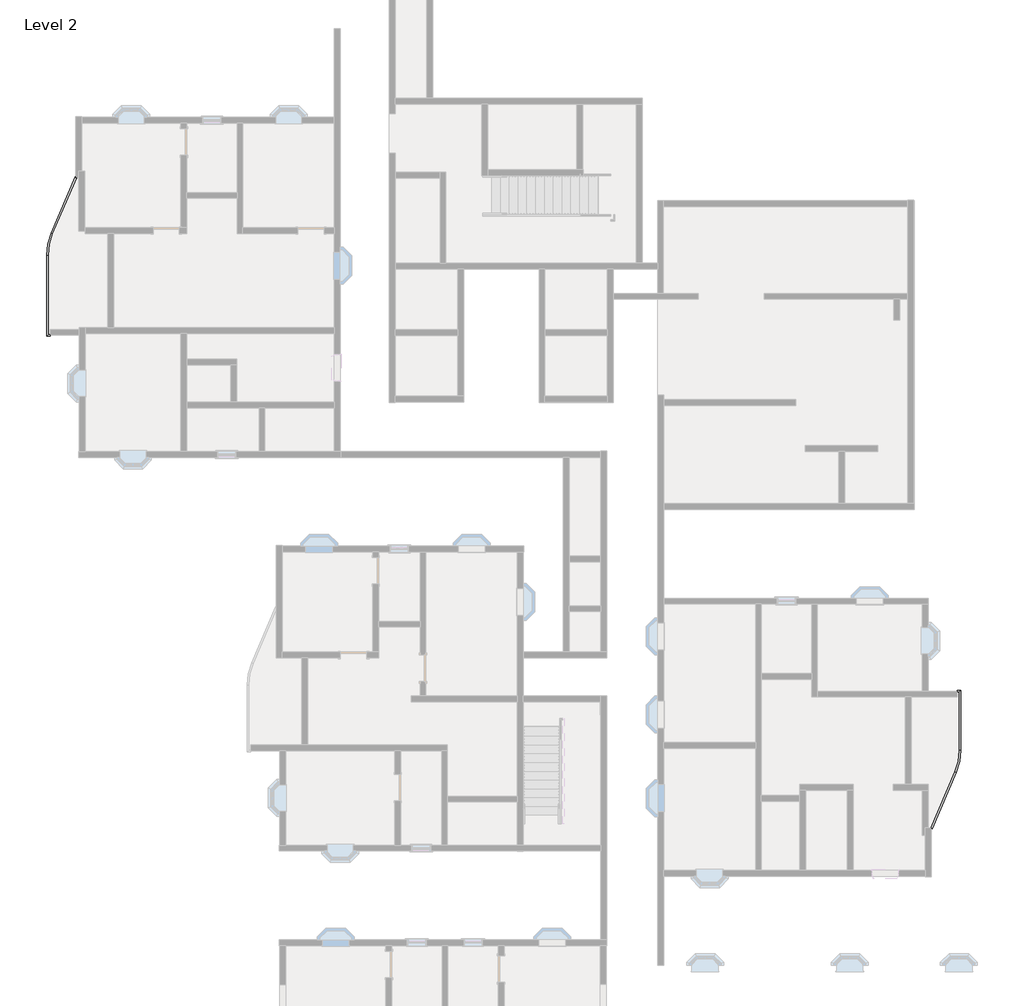
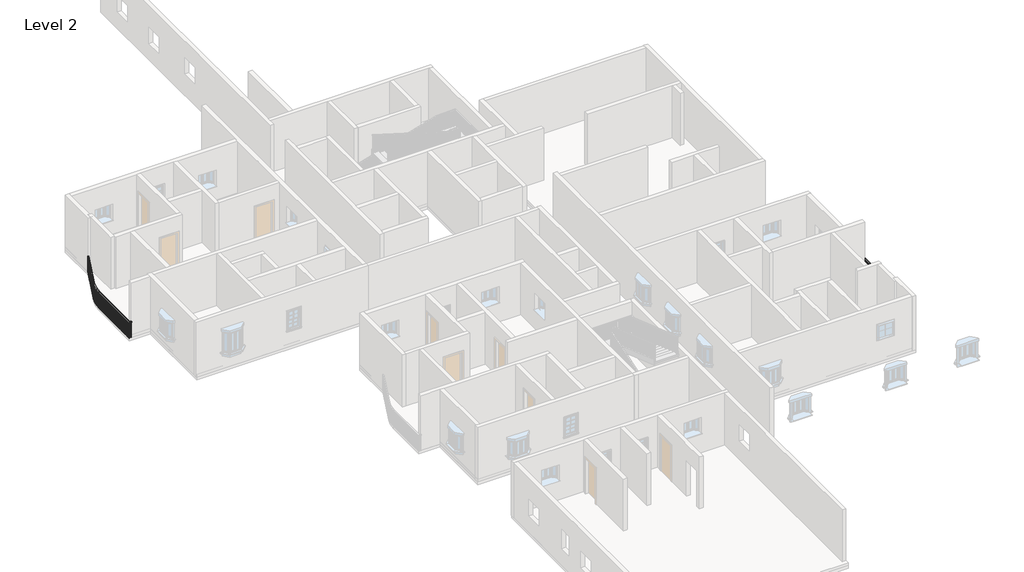
# One storey, part 9 of 14: 2 railings.
"""IFC4 building model written with IfcOpenShell, lengths in millimetres."""

from ifc_helpers import new_model, si_unit, frame, origin, place, context, project, spatial, polyline, circle_curve, outline, extrude, element, save
from ifc_brep_helpers import plane_surface, cylinder_surface, revolved_surface, advanced_brep

model = new_model("IFC4")

# Units and contexts
model_context = context("Model", 3, world=origin())
ifc_project = project(units=[si_unit("LENGTHUNIT", "METRE", prefix="MILLI")], contexts=[model_context])

# Site, building, storey
site = spatial("IfcSite", under=ifc_project)
building = spatial("IfcBuilding", under=site)
storey = spatial("IfcBuildingStorey", under=building, Name="Level 2", Elevation=3048.0)

# Railings
placement = place(None, origin())
element("IfcRailing", 1, ObjectType="Handrail - Rectangular", at=placement, inside=storey, context=model_context, shape_type="SolidModel", body=[
    advanced_brep(
    [(-19327.739878, 12446.0257339, 3962.4), (-19327.739878, 12446.0257339, 3911.6), (-19374.4383922, 12466.022953, 3911.6), (-19374.4383922, 12466.022953, 3962.4), (-20162.483418, 10496.6905323, 3962.4), (-20162.483418, 10496.6905323, 3911.6), (-20209.1819322, 10516.6877514, 3911.6), (-20209.1819322, 10516.6877514, 3962.4), (-20316.2891351, 9746.7948172, 3911.6), (-20316.2891351, 9746.7948172, 3962.4), (-20367.0891351, 9746.7948172, 3911.6), (-20367.0891351, 9746.7948172, 3962.4), (-20316.2891351, 7005.2583494, 3962.4), (-20316.2891351, 7005.2583494, 3911.6), (-20367.0891351, 6954.4583494, 3911.6), (-20367.0891351, 6954.4583494, 3962.4), (-20240.0891351, 7005.2583494, 3962.4), (-20240.0891351, 6954.4583494, 3962.4), (-20240.0891351, 6954.4583494, 3911.6), (-20240.0891351, 7005.2583494, 3911.6)],
    [
        (0, 1),
        (1, 2),
        (2, 3),
        (3, 0),
        (0, 4),
        (4, 5),
        (5, 1),
        (5, 6),
        (6, 2),
        (6, 7),
        (7, 3),
        (7, 4),
        (8, 5, circle_curve(frame((-18411.2891351, 9746.7948172, 3911.6), z_axis=(0.0, 0.0, -1.0), x_axis=(-0.9192620907623915, 0.3936460446735831, 0.0)), 1905.0)),
        (4, 9, circle_curve(frame((-18411.2891351, 9746.7948172, 3962.4), z_axis=(0.0, 0.0, 1.0), x_axis=(-0.9192620907623915, 0.3936460446735831, 0.0)), 1905.0)),
        (9, 8),
        (10, 6, circle_curve(frame((-18411.2891351, 9746.7948172, 3911.6), z_axis=(0.0, 0.0, -1.0), x_axis=(-0.9192620907623915, 0.3936460446735831, 0.0)), 1955.8)),
        (8, 10),
        (11, 7, circle_curve(frame((-18411.2891351, 9746.7948172, 3962.4), z_axis=(0.0, 0.0, -1.0), x_axis=(-0.9192620907623915, 0.3936460446735831, 0.0)), 1955.8)),
        (10, 11),
        (11, 9),
        (9, 12),
        (12, 13),
        (13, 8),
        (13, 14),
        (14, 10),
        (14, 15),
        (15, 11),
        (15, 12),
        (16, 17),
        (17, 18),
        (18, 19),
        (19, 16),
        (12, 16),
        (19, 13),
        (18, 14),
        (17, 15),
    ],
    [
        plane_surface(frame((-19351.0891351, 12456.0243434, 3962.4), z_axis=(0.3936460446735829, 0.9192620907623917, 0.0), x_axis=(0.9192620907623917, -0.3936460446735829, 0.0))),
        plane_surface(frame((-19327.739878, 12446.0257339, 3962.4), z_axis=(0.9192620907623913, -0.3936460446735837, 0.0), x_axis=(-0.3936460446735837, -0.9192620907623913, 0.0))),
        plane_surface(frame((-19327.739878, 12446.0257339, 3911.6), z_axis=(0.0, 0.0, -1.0), x_axis=(-0.3936460446735837, -0.9192620907623913, 0.0))),
        plane_surface(frame((-19374.4383922, 12466.022953, 3911.6), z_axis=(-0.9192620907623915, 0.3936460446735834, 0.0), x_axis=(-0.3936460446735834, -0.9192620907623915, 0.0))),
        plane_surface(frame((-19374.4383922, 12466.022953, 3962.4), z_axis=(0.0, 0.0, 1.0000000000000002), x_axis=(-0.3936460446735834, -0.9192620907623915, 0.0))),
        revolved_surface(polyline([(-20162.483418002357, 10496.690532303175, 3962.4), (-20162.483418002357, 10496.690532303175, 3911.6)]), (-18411.2891351, 9746.7948172, 3962.4), (0.0, 0.0, 1.0)),
        plane_surface(frame((-18411.2891351, 9746.7948172, 3911.6), z_axis=(0.0, 0.0, -1.0000000000000002), x_axis=(-0.9192620907623916, 0.39364604467358316, 0.0))),
        cylinder_surface(frame((-18411.2891351, 9746.7948172, 3962.4), z_axis=(0.0, 0.0, 1.0), x_axis=(-0.9192620907623915, 0.3936460446735831, 0.0)), 1955.8),
        plane_surface(frame((-18411.2891351, 9746.7948172, 3962.4), z_axis=(0.0, 0.0, 1.0000000000000002), x_axis=(-0.9192620907623916, 0.39364604467358316, 0.0))),
        plane_surface(frame((-20316.2891351, 9746.7948172, 3962.4), z_axis=(1.0, 0.0, 0.0), x_axis=(0.0, -1.0, 0.0))),
        plane_surface(frame((-20316.2891351, 9746.7948172, 3911.6), z_axis=(0.0, 0.0, -1.0), x_axis=(0.0, -1.0, 0.0))),
        plane_surface(frame((-20367.0891351, 9746.7948172, 3911.6), z_axis=(-1.0, 0.0, 0.0), x_axis=(0.0, -1.0, 0.0))),
        plane_surface(frame((-20367.0891351, 9746.7948172, 3962.4), z_axis=(0.0, 0.0, 1.0), x_axis=(0.0, -1.0, 0.0))),
        plane_surface(frame((-20240.0891351, 6979.8583494, 3962.4), z_axis=(1.0, 0.0, 0.0), x_axis=(0.0, 1.0, 0.0))),
        plane_surface(frame((-20316.2891351, 7005.2583494, 3962.4), z_axis=(0.0, 1.0, 0.0), x_axis=(1.0, 0.0, 0.0))),
        plane_surface(frame((-20316.2891351, 7005.2583494, 3911.6), z_axis=(0.0, 0.0, -1.0), x_axis=(1.0, 0.0, 0.0))),
        plane_surface(frame((-20367.0891351, 6954.4583494, 3911.6), z_axis=(0.0, -1.0, 0.0), x_axis=(1.0, 0.0, 0.0))),
        plane_surface(frame((-20367.0891351, 6954.4583494, 3962.4), z_axis=(0.0, 0.0, 1.0), x_axis=(1.0, 0.0, 0.0))),
    ],
    [
        (0, [[1, 2, 3, 4]]),
        (1, [[-1, 5, 6, 7]]),
        (2, [[-2, -7, 8, 9]]),
        (3, [[-3, -9, 10, 11]]),
        (4, [[-4, -11, 12, -5]]),
        (5, [[13, -6, 14, 15]]),
        (6, [[16, -8, -13, 17]]),
        (7, [[18, -10, -16, 19]]),
        (8, [[-14, -12, -18, 20]]),
        (9, [[-15, 21, 22, 23]]),
        (10, [[-17, -23, 24, 25]]),
        (11, [[-19, -25, 26, 27]]),
        (12, [[-20, -27, 28, -21]]),
        (13, [[29, 30, 31, 32]]),
        (14, [[-22, 33, -32, 34]]),
        (15, [[-24, -34, -31, 35]]),
        (16, [[-26, -35, -30, 36]]),
        (17, [[-28, -36, -29, -33]]),
    ],
),
    extrude(outline(polyline([(-20351.2141351, 7013.1198172), (-20332.1641351, 7013.1198172), (-20332.1641351, 6994.0698172), (-20351.2141351, 6994.0698172), (-20351.2141351, 7013.1198172)])), frame((0.0, 0.0, 3048.0), z_axis=(0.0, 0.0, 1.0), x_axis=(1.0, 0.0, 0.0)), (0.0, 0.0, 1.0), 863.6),
    extrude(outline(polyline([(-20351.2141351, 7114.7198172), (-20332.1641351, 7114.7198172), (-20332.1641351, 7095.6698172), (-20351.2141351, 7095.6698172), (-20351.2141351, 7114.7198172)])), frame((0.0, 0.0, 3048.0), z_axis=(0.0, 0.0, 1.0), x_axis=(1.0, 0.0, 0.0)), (0.0, 0.0, 1.0), 863.6),
    extrude(outline(polyline([(-20351.2141351, 7216.3198172), (-20332.1641351, 7216.3198172), (-20332.1641351, 7197.2698172), (-20351.2141351, 7197.2698172), (-20351.2141351, 7216.3198172)])), frame((0.0, 0.0, 3048.0), z_axis=(0.0, 0.0, 1.0), x_axis=(1.0, 0.0, 0.0)), (0.0, 0.0, 1.0), 863.6),
    extrude(outline(polyline([(-20351.2141351, 7317.9198172), (-20332.1641351, 7317.9198172), (-20332.1641351, 7298.8698172), (-20351.2141351, 7298.8698172), (-20351.2141351, 7317.9198172)])), frame((0.0, 0.0, 3048.0), z_axis=(0.0, 0.0, 1.0), x_axis=(1.0, 0.0, 0.0)), (0.0, 0.0, 1.0), 863.6),
    extrude(outline(polyline([(-20351.2141351, 7419.5198172), (-20332.1641351, 7419.5198172), (-20332.1641351, 7400.4698172), (-20351.2141351, 7400.4698172), (-20351.2141351, 7419.5198172)])), frame((0.0, 0.0, 3048.0), z_axis=(0.0, 0.0, 1.0), x_axis=(1.0, 0.0, 0.0)), (0.0, 0.0, 1.0), 863.6),
    extrude(outline(polyline([(-20351.2141351, 7521.1198172), (-20332.1641351, 7521.1198172), (-20332.1641351, 7502.0698172), (-20351.2141351, 7502.0698172), (-20351.2141351, 7521.1198172)])), frame((0.0, 0.0, 3048.0), z_axis=(0.0, 0.0, 1.0), x_axis=(1.0, 0.0, 0.0)), (0.0, 0.0, 1.0), 863.6),
    extrude(outline(polyline([(-20351.2141351, 7622.7198172), (-20332.1641351, 7622.7198172), (-20332.1641351, 7603.6698172), (-20351.2141351, 7603.6698172), (-20351.2141351, 7622.7198172)])), frame((0.0, 0.0, 3048.0), z_axis=(0.0, 0.0, 1.0), x_axis=(1.0, 0.0, 0.0)), (0.0, 0.0, 1.0), 863.6),
    extrude(outline(polyline([(-20351.2141351, 7724.3198172), (-20332.1641351, 7724.3198172), (-20332.1641351, 7705.2698172), (-20351.2141351, 7705.2698172), (-20351.2141351, 7724.3198172)])), frame((0.0, 0.0, 3048.0), z_axis=(0.0, 0.0, 1.0), x_axis=(1.0, 0.0, 0.0)), (0.0, 0.0, 1.0), 863.6),
    extrude(outline(polyline([(-20351.2141351, 7825.9198172), (-20332.1641351, 7825.9198172), (-20332.1641351, 7806.8698172), (-20351.2141351, 7806.8698172), (-20351.2141351, 7825.9198172)])), frame((0.0, 0.0, 3048.0), z_axis=(0.0, 0.0, 1.0), x_axis=(1.0, 0.0, 0.0)), (0.0, 0.0, 1.0), 863.6),
    extrude(outline(polyline([(-20351.2141351, 7927.5198172), (-20332.1641351, 7927.5198172), (-20332.1641351, 7908.4698172), (-20351.2141351, 7908.4698172), (-20351.2141351, 7927.5198172)])), frame((0.0, 0.0, 3048.0), z_axis=(0.0, 0.0, 1.0), x_axis=(1.0, 0.0, 0.0)), (0.0, 0.0, 1.0), 863.6),
    extrude(outline(polyline([(-20351.2141351, 8029.1198172), (-20332.1641351, 8029.1198172), (-20332.1641351, 8010.0698172), (-20351.2141351, 8010.0698172), (-20351.2141351, 8029.1198172)])), frame((0.0, 0.0, 3048.0), z_axis=(0.0, 0.0, 1.0), x_axis=(1.0, 0.0, 0.0)), (0.0, 0.0, 1.0), 863.6),
    extrude(outline(polyline([(-20351.2141351, 8130.7198172), (-20332.1641351, 8130.7198172), (-20332.1641351, 8111.6698172), (-20351.2141351, 8111.6698172), (-20351.2141351, 8130.7198172)])), frame((0.0, 0.0, 3048.0), z_axis=(0.0, 0.0, 1.0), x_axis=(1.0, 0.0, 0.0)), (0.0, 0.0, 1.0), 863.6),
    extrude(outline(polyline([(-20351.2141351, 8232.3198172), (-20332.1641351, 8232.3198172), (-20332.1641351, 8213.2698172), (-20351.2141351, 8213.2698172), (-20351.2141351, 8232.3198172)])), frame((0.0, 0.0, 3048.0), z_axis=(0.0, 0.0, 1.0), x_axis=(1.0, 0.0, 0.0)), (0.0, 0.0, 1.0), 863.6),
    extrude(outline(polyline([(-20351.2141351, 8333.9198172), (-20332.1641351, 8333.9198172), (-20332.1641351, 8314.8698172), (-20351.2141351, 8314.8698172), (-20351.2141351, 8333.9198172)])), frame((0.0, 0.0, 3048.0), z_axis=(0.0, 0.0, 1.0), x_axis=(1.0, 0.0, 0.0)), (0.0, 0.0, 1.0), 863.6),
    extrude(outline(polyline([(-20351.2141351, 8435.5198172), (-20332.1641351, 8435.5198172), (-20332.1641351, 8416.4698172), (-20351.2141351, 8416.4698172), (-20351.2141351, 8435.5198172)])), frame((0.0, 0.0, 3048.0), z_axis=(0.0, 0.0, 1.0), x_axis=(1.0, 0.0, 0.0)), (0.0, 0.0, 1.0), 863.6),
    extrude(outline(polyline([(-20351.2141351, 8537.1198172), (-20332.1641351, 8537.1198172), (-20332.1641351, 8518.0698172), (-20351.2141351, 8518.0698172), (-20351.2141351, 8537.1198172)])), frame((0.0, 0.0, 3048.0), z_axis=(0.0, 0.0, 1.0), x_axis=(1.0, 0.0, 0.0)), (0.0, 0.0, 1.0), 863.6),
    extrude(outline(polyline([(-20351.2141351, 8638.7198172), (-20332.1641351, 8638.7198172), (-20332.1641351, 8619.6698172), (-20351.2141351, 8619.6698172), (-20351.2141351, 8638.7198172)])), frame((0.0, 0.0, 3048.0), z_axis=(0.0, 0.0, 1.0), x_axis=(1.0, 0.0, 0.0)), (0.0, 0.0, 1.0), 863.6),
    extrude(outline(polyline([(-20351.2141351, 8740.3198172), (-20332.1641351, 8740.3198172), (-20332.1641351, 8721.2698172), (-20351.2141351, 8721.2698172), (-20351.2141351, 8740.3198172)])), frame((0.0, 0.0, 3048.0), z_axis=(0.0, 0.0, 1.0), x_axis=(1.0, 0.0, 0.0)), (0.0, 0.0, 1.0), 863.6),
    extrude(outline(polyline([(-20351.2141351, 8841.9198172), (-20332.1641351, 8841.9198172), (-20332.1641351, 8822.8698172), (-20351.2141351, 8822.8698172), (-20351.2141351, 8841.9198172)])), frame((0.0, 0.0, 3048.0), z_axis=(0.0, 0.0, 1.0), x_axis=(1.0, 0.0, 0.0)), (0.0, 0.0, 1.0), 863.6),
    extrude(outline(polyline([(-20351.2141351, 8943.5198172), (-20332.1641351, 8943.5198172), (-20332.1641351, 8924.4698172), (-20351.2141351, 8924.4698172), (-20351.2141351, 8943.5198172)])), frame((0.0, 0.0, 3048.0), z_axis=(0.0, 0.0, 1.0), x_axis=(1.0, 0.0, 0.0)), (0.0, 0.0, 1.0), 863.6),
    extrude(outline(polyline([(-20351.2141351, 9045.1198172), (-20332.1641351, 9045.1198172), (-20332.1641351, 9026.0698172), (-20351.2141351, 9026.0698172), (-20351.2141351, 9045.1198172)])), frame((0.0, 0.0, 3048.0), z_axis=(0.0, 0.0, 1.0), x_axis=(1.0, 0.0, 0.0)), (0.0, 0.0, 1.0), 863.6),
    extrude(outline(polyline([(-20351.2141351, 9146.7198172), (-20332.1641351, 9146.7198172), (-20332.1641351, 9127.6698172), (-20351.2141351, 9127.6698172), (-20351.2141351, 9146.7198172)])), frame((0.0, 0.0, 3048.0), z_axis=(0.0, 0.0, 1.0), x_axis=(1.0, 0.0, 0.0)), (0.0, 0.0, 1.0), 863.6),
    extrude(outline(polyline([(-20351.2141351, 9248.3198172), (-20332.1641351, 9248.3198172), (-20332.1641351, 9229.2698172), (-20351.2141351, 9229.2698172), (-20351.2141351, 9248.3198172)])), frame((0.0, 0.0, 3048.0), z_axis=(0.0, 0.0, 1.0), x_axis=(1.0, 0.0, 0.0)), (0.0, 0.0, 1.0), 863.6),
    extrude(outline(polyline([(-20351.2141351, 9349.9198172), (-20332.1641351, 9349.9198172), (-20332.1641351, 9330.8698172), (-20351.2141351, 9330.8698172), (-20351.2141351, 9349.9198172)])), frame((0.0, 0.0, 3048.0), z_axis=(0.0, 0.0, 1.0), x_axis=(1.0, 0.0, 0.0)), (0.0, 0.0, 1.0), 863.6),
    extrude(outline(polyline([(-20351.2141351, 9451.5198172), (-20332.1641351, 9451.5198172), (-20332.1641351, 9432.4698172), (-20351.2141351, 9432.4698172), (-20351.2141351, 9451.5198172)])), frame((0.0, 0.0, 3048.0), z_axis=(0.0, 0.0, 1.0), x_axis=(1.0, 0.0, 0.0)), (0.0, 0.0, 1.0), 863.6),
    extrude(outline(polyline([(-20351.2141351, 9553.1198172), (-20332.1641351, 9553.1198172), (-20332.1641351, 9534.0698172), (-20351.2141351, 9534.0698172), (-20351.2141351, 9553.1198172)])), frame((0.0, 0.0, 3048.0), z_axis=(0.0, 0.0, 1.0), x_axis=(1.0, 0.0, 0.0)), (0.0, 0.0, 1.0), 863.6),
    extrude(outline(polyline([(-20351.2141351, 9654.7198172), (-20332.1641351, 9654.7198172), (-20332.1641351, 9635.6698172), (-20351.2141351, 9635.6698172), (-20351.2141351, 9654.7198172)])), frame((0.0, 0.0, 3048.0), z_axis=(0.0, 0.0, 1.0), x_axis=(1.0, 0.0, 0.0)), (0.0, 0.0, 1.0), 863.6),
    extrude(outline(polyline([(-20349.6005818, 9826.4720848), (-20330.5630441, 9825.7831307), (-20331.2519982, 9806.745593), (-20350.289536, 9807.4345471), (-20349.6005818, 9826.4720848)])), frame((0.0, 0.0, 3048.0), z_axis=(0.0, 0.0, 1.0), x_axis=(1.0, 0.0, 0.0)), (0.0, 0.0, 1.0), 863.6),
    extrude(outline(polyline([(-20342.724955, 9928.3310534), (-20323.750023, 9926.6415402), (-20325.4395363, 9907.6666081), (-20344.4144683, 9909.3561214), (-20342.724955, 9928.3310534)])), frame((0.0, 0.0, 3048.0), z_axis=(0.0, 0.0, 1.0), x_axis=(1.0, 0.0, 0.0)), (0.0, 0.0, 1.0), 863.6),
    extrude(outline(polyline([(-20330.5003254, 10029.6872677), (-20311.6405491, 10027.0018743), (-20314.3259425, 10008.142098), (-20333.1857188, 10010.8274914), (-20330.5003254, 10029.6872677)])), frame((0.0, 0.0, 3048.0), z_axis=(0.0, 0.0, 1.0), x_axis=(1.0, 0.0, 0.0)), (0.0, 0.0, 1.0), 863.6),
    extrude(outline(polyline([(-20312.9605484, 10130.2600272), (-20294.2681589, 10126.5861907), (-20297.9419954, 10107.8938012), (-20316.6343849, 10111.5676377), (-20312.9605484, 10130.2600272)])), frame((0.0, 0.0, 3048.0), z_axis=(0.0, 0.0, 1.0), x_axis=(1.0, 0.0, 0.0)), (0.0, 0.0, 1.0), 863.6),
    extrude(outline(polyline([(-20290.1541995, 10229.7708014), (-20271.6809643, 10225.1186963), (-20276.3330693, 10206.6454611), (-20294.8063045, 10211.2975662), (-20290.1541995, 10229.7708014)])), frame((0.0, 0.0, 3048.0), z_axis=(0.0, 0.0, 1.0), x_axis=(1.0, 0.0, 0.0)), (0.0, 0.0, 1.0), 863.6),
    extrude(outline(polyline([(-20262.1444395, 10327.9440008), (-20243.9415192, 10322.3265109), (-20249.5590091, 10304.1235906), (-20267.7619294, 10309.7410805), (-20262.1444395, 10327.9440008)])), frame((0.0, 0.0, 3048.0), z_axis=(0.0, 0.0, 1.0), x_axis=(1.0, 0.0, 0.0)), (0.0, 0.0, 1.0), 863.6),
    extrude(outline(polyline([(-20229.0088399, 10424.5077402), (-20211.1266465, 10417.9404228), (-20217.693964, 10400.0582293), (-20235.5761574, 10406.6255468), (-20229.0088399, 10424.5077402)])), frame((0.0, 0.0, 3048.0), z_axis=(0.0, 0.0, 1.0), x_axis=(1.0, 0.0, 0.0)), (0.0, 0.0, 1.0), 863.6),
    extrude(outline(polyline([(-20155.9843907, 10600.589225), (-20138.4724479, 10593.0902678), (-20145.9714051, 10575.578325), (-20163.4833479, 10583.0772822), (-20155.9843907, 10600.589225)])), frame((0.0, 0.0, 3048.0), z_axis=(0.0, 0.0, 1.0), x_axis=(1.0, 0.0, 0.0)), (0.0, 0.0, 1.0), 863.6),
    extrude(outline(polyline([(-20115.9899526, 10693.9862534), (-20098.4780098, 10686.4872963), (-20105.9769669, 10668.9753534), (-20123.4889098, 10676.4743106), (-20115.9899526, 10693.9862534)])), frame((0.0, 0.0, 3048.0), z_axis=(0.0, 0.0, 1.0), x_axis=(1.0, 0.0, 0.0)), (0.0, 0.0, 1.0), 863.6),
    extrude(outline(polyline([(-20075.9955145, 10787.3832818), (-20058.4835716, 10779.8843247), (-20065.9825288, 10762.3723818), (-20083.4944716, 10769.871339), (-20075.9955145, 10787.3832818)])), frame((0.0, 0.0, 3048.0), z_axis=(0.0, 0.0, 1.0), x_axis=(1.0, 0.0, 0.0)), (0.0, 0.0, 1.0), 863.6),
    extrude(outline(polyline([(-20036.0010763, 10880.7803103), (-20018.4891335, 10873.2813531), (-20025.9880906, 10855.7694103), (-20043.5000335, 10863.2683674), (-20036.0010763, 10880.7803103)])), frame((0.0, 0.0, 3048.0), z_axis=(0.0, 0.0, 1.0), x_axis=(1.0, 0.0, 0.0)), (0.0, 0.0, 1.0), 863.6),
    extrude(outline(polyline([(-19996.0066382, 10974.1773387), (-19978.4946954, 10966.6783815), (-19985.9936525, 10949.1664387), (-20003.5055953, 10956.6653958), (-19996.0066382, 10974.1773387)])), frame((0.0, 0.0, 3048.0), z_axis=(0.0, 0.0, 1.0), x_axis=(1.0, 0.0, 0.0)), (0.0, 0.0, 1.0), 863.6),
    extrude(outline(polyline([(-19956.0122, 11067.5743671), (-19938.5002572, 11060.0754099), (-19945.9992144, 11042.5634671), (-19963.5111572, 11050.0624243), (-19956.0122, 11067.5743671)])), frame((0.0, 0.0, 3048.0), z_axis=(0.0, 0.0, 1.0), x_axis=(1.0, 0.0, 0.0)), (0.0, 0.0, 1.0), 863.6),
    extrude(outline(polyline([(-19916.0177619, 11160.9713955), (-19898.5058191, 11153.4724384), (-19906.0047762, 11135.9604955), (-19923.5167191, 11143.4594527), (-19916.0177619, 11160.9713955)])), frame((0.0, 0.0, 3048.0), z_axis=(0.0, 0.0, 1.0), x_axis=(1.0, 0.0, 0.0)), (0.0, 0.0, 1.0), 863.6),
    extrude(outline(polyline([(-19876.0233238, 11254.3684239), (-19858.5113809, 11246.8694668), (-19866.0103381, 11229.357524), (-19883.5222809, 11236.8564811), (-19876.0233238, 11254.3684239)])), frame((0.0, 0.0, 3048.0), z_axis=(0.0, 0.0, 1.0), x_axis=(1.0, 0.0, 0.0)), (0.0, 0.0, 1.0), 863.6),
    extrude(outline(polyline([(-19836.0288856, 11347.7654524), (-19818.5169428, 11340.2664952), (-19826.0159, 11322.7545524), (-19843.5278428, 11330.2535095), (-19836.0288856, 11347.7654524)])), frame((0.0, 0.0, 3048.0), z_axis=(0.0, 0.0, 1.0), x_axis=(1.0, 0.0, 0.0)), (0.0, 0.0, 1.0), 863.6),
    extrude(outline(polyline([(-19796.0344475, 11441.1624808), (-19778.5225047, 11433.6635236), (-19786.0214618, 11416.1515808), (-19803.5334046, 11423.650538), (-19796.0344475, 11441.1624808)])), frame((0.0, 0.0, 3048.0), z_axis=(0.0, 0.0, 1.0), x_axis=(1.0, 0.0, 0.0)), (0.0, 0.0, 1.0), 863.6),
    extrude(outline(polyline([(-19756.0400094, 11534.5595092), (-19738.5280665, 11527.060552), (-19746.0270237, 11509.5486092), (-19763.5389665, 11517.0475664), (-19756.0400094, 11534.5595092)])), frame((0.0, 0.0, 3048.0), z_axis=(0.0, 0.0, 1.0), x_axis=(1.0, 0.0, 0.0)), (0.0, 0.0, 1.0), 863.6),
    extrude(outline(polyline([(-19716.0455712, 11627.9565376), (-19698.5336284, 11620.4575805), (-19706.0325855, 11602.9456376), (-19723.5445284, 11610.4445948), (-19716.0455712, 11627.9565376)])), frame((0.0, 0.0, 3048.0), z_axis=(0.0, 0.0, 1.0), x_axis=(1.0, 0.0, 0.0)), (0.0, 0.0, 1.0), 863.6),
    extrude(outline(polyline([(-19676.0511331, 11721.353566), (-19658.5391902, 11713.8546089), (-19666.0381474, 11696.3426661), (-19683.5500902, 11703.8416232), (-19676.0511331, 11721.353566)])), frame((0.0, 0.0, 3048.0), z_axis=(0.0, 0.0, 1.0), x_axis=(1.0, 0.0, 0.0)), (0.0, 0.0, 1.0), 863.6),
    extrude(outline(polyline([(-19636.0566949, 11814.7505945), (-19618.5447521, 11807.2516373), (-19626.0437093, 11789.7396945), (-19643.5556521, 11797.2386516), (-19636.0566949, 11814.7505945)])), frame((0.0, 0.0, 3048.0), z_axis=(0.0, 0.0, 1.0), x_axis=(1.0, 0.0, 0.0)), (0.0, 0.0, 1.0), 863.6),
    extrude(outline(polyline([(-19596.0622568, 11908.1476229), (-19578.550314, 11900.6486657), (-19586.0492711, 11883.1367229), (-19603.561214, 11890.6356801), (-19596.0622568, 11908.1476229)])), frame((0.0, 0.0, 3048.0), z_axis=(0.0, 0.0, 1.0), x_axis=(1.0, 0.0, 0.0)), (0.0, 0.0, 1.0), 863.6),
    extrude(outline(polyline([(-19556.0678187, 12001.5446513), (-19538.5558758, 11994.0456942), (-19546.054833, 11976.5337513), (-19563.5667758, 11984.0327085), (-19556.0678187, 12001.5446513)])), frame((0.0, 0.0, 3048.0), z_axis=(0.0, 0.0, 1.0), x_axis=(1.0, 0.0, 0.0)), (0.0, 0.0, 1.0), 863.6),
    extrude(outline(polyline([(-19516.0733805, 12094.9416797), (-19498.5614377, 12087.4427226), (-19506.0603948, 12069.9307797), (-19523.5723377, 12077.4297369), (-19516.0733805, 12094.9416797)])), frame((0.0, 0.0, 3048.0), z_axis=(0.0, 0.0, 1.0), x_axis=(1.0, 0.0, 0.0)), (0.0, 0.0, 1.0), 863.6),
    extrude(outline(polyline([(-19476.0789424, 12188.3387082), (-19458.5669996, 12180.839751), (-19466.0659567, 12163.3278082), (-19483.5778995, 12170.8267653), (-19476.0789424, 12188.3387082)])), frame((0.0, 0.0, 3048.0), z_axis=(0.0, 0.0, 1.0), x_axis=(1.0, 0.0, 0.0)), (0.0, 0.0, 1.0), 863.6),
    extrude(outline(polyline([(-19436.0845042, 12281.7357366), (-19418.5725614, 12274.2367794), (-19426.0715186, 12256.7248366), (-19443.5834614, 12264.2237937), (-19436.0845042, 12281.7357366)])), frame((0.0, 0.0, 3048.0), z_axis=(0.0, 0.0, 1.0), x_axis=(1.0, 0.0, 0.0)), (0.0, 0.0, 1.0), 863.6),
    extrude(outline(polyline([(-19396.0900661, 12375.132765), (-19378.5781233, 12367.6338078), (-19386.0770804, 12350.121865), (-19403.5890233, 12357.6208222), (-19396.0900661, 12375.132765)])), frame((0.0, 0.0, 3048.0), z_axis=(0.0, 0.0, 1.0), x_axis=(1.0, 0.0, 0.0)), (0.0, 0.0, 1.0), 863.6),
    extrude(outline(polyline([(-20351.2141351, 6989.3833494), (-20332.1641351, 6989.3833494), (-20332.1641351, 6970.3333494), (-20351.2141351, 6970.3333494), (-20351.2141351, 6989.3833494)])), frame((0.0, 0.0, 3048.0), z_axis=(0.0, 0.0, 1.0), x_axis=(1.0, 0.0, 0.0)), (0.0, 0.0, 1.0), 863.6),
    extrude(outline(polyline([(-20351.2141351, 9756.3198172), (-20332.1641351, 9756.3198172), (-20332.1641351, 9737.2698172), (-20351.2141351, 9737.2698172), (-20351.2141351, 9756.3198172)])), frame((0.0, 0.0, 3048.0), z_axis=(0.0, 0.0, 1.0), x_axis=(1.0, 0.0, 0.0)), (0.0, 0.0, 1.0), 863.6),
    extrude(outline(polyline([(-20190.839168, 10519.1945919), (-20173.3272251, 10511.6956347), (-20180.8261823, 10494.1836919), (-20198.3381251, 10501.682649), (-20190.839168, 10519.1945919)])), frame((0.0, 0.0, 3048.0), z_axis=(0.0, 0.0, 1.0), x_axis=(1.0, 0.0, 0.0)), (0.0, 0.0, 1.0), 863.6),
    extrude(outline(polyline([(-20259.1391351, 6970.3333494), (-20259.1391351, 6989.3833494), (-20240.0891351, 6989.3833494), (-20240.0891351, 6970.3333494), (-20259.1391351, 6970.3333494)])), frame((0.0, 0.0, 3048.0), z_axis=(0.0, 0.0, 1.0), x_axis=(1.0, 0.0, 0.0)), (0.0, 0.0, 1.0), 863.6),
    extrude(outline(polyline([(-19359.8451065, 12459.773822), (-19342.3331637, 12452.2748648), (-19349.8321209, 12434.762922), (-19367.3440637, 12442.2618792), (-19359.8451065, 12459.773822)])), frame((0.0, 0.0, 3048.0), z_axis=(0.0, 0.0, 1.0), x_axis=(1.0, 0.0, 0.0)), (0.0, 0.0, 1.0), 863.6),
])
element("IfcRailing", 2, ObjectType="Handrail - Rectangular", at=placement, inside=storey, context=model_context, shape_type="SolidModel", body=[
    advanced_brep(
    [(10250.7887952, -10096.81198, 3962.4), (10250.7887952, -10096.81198, 3911.6), (10297.4873094, -10116.8091991, 3911.6), (10297.4873094, -10116.8091991, 3962.4), (11085.5323352, -8147.4767784, 3962.4), (11085.5323352, -8147.4767784, 3911.6), (11132.2308494, -8167.4739975, 3911.6), (11132.2308494, -8167.4739975, 3962.4), (11239.3380523, -7397.5810633, 3911.6), (11239.3380523, -7397.5810633, 3962.4), (11290.1380523, -7397.5810633, 3911.6), (11290.1380523, -7397.5810633, 3962.4), (11239.3380523, -5378.0542694, 3962.4), (11239.3380523, -5378.0542694, 3911.6), (11290.1380523, -5327.2542694, 3911.6), (11290.1380523, -5327.2542694, 3962.4), (11163.1380523, -5378.0542694, 3962.4), (11163.1380523, -5327.2542694, 3962.4), (11163.1380523, -5327.2542694, 3911.6), (11163.1380523, -5378.0542694, 3911.6)],
    [
        (0, 1),
        (1, 2),
        (2, 3),
        (3, 0),
        (0, 4),
        (4, 5),
        (5, 1),
        (5, 6),
        (6, 2),
        (6, 7),
        (7, 3),
        (7, 4),
        (8, 5, circle_curve(frame((9334.3380523, -7397.5810633, 3911.6), z_axis=(0.0, 0.0, -1.0), x_axis=(0.9192620907624003, -0.3936460446735628, 0.0)), 1905.0)),
        (4, 9, circle_curve(frame((9334.3380523, -7397.5810633, 3962.4), z_axis=(0.0, 0.0, 1.0), x_axis=(0.9192620907624003, -0.3936460446735628, 0.0)), 1905.0)),
        (9, 8),
        (10, 6, circle_curve(frame((9334.3380523, -7397.5810633, 3911.6), z_axis=(0.0, 0.0, -1.0), x_axis=(0.9192620907624003, -0.3936460446735628, 0.0)), 1955.8)),
        (8, 10),
        (11, 7, circle_curve(frame((9334.3380523, -7397.5810633, 3962.4), z_axis=(0.0, 0.0, -1.0), x_axis=(0.9192620907624003, -0.3936460446735628, 0.0)), 1955.8)),
        (10, 11),
        (11, 9),
        (9, 12),
        (12, 13),
        (13, 8),
        (13, 14),
        (14, 10),
        (14, 15),
        (15, 11),
        (15, 12),
        (16, 17),
        (17, 18),
        (18, 19),
        (19, 16),
        (12, 16),
        (19, 13),
        (18, 14),
        (17, 15),
    ],
    [
        plane_surface(frame((10274.1380523, -10106.8105895, 3962.4), z_axis=(-0.3936460446735629, -0.9192620907624003, 0.0), x_axis=(0.9192620907624003, -0.3936460446735629, 0.0))),
        plane_surface(frame((10250.7887952, -10096.81198, 3962.4), z_axis=(-0.9192620907624004, 0.3936460446735625, 0.0), x_axis=(0.3936460446735625, 0.9192620907624004, 0.0))),
        plane_surface(frame((10250.7887952, -10096.81198, 3911.6), z_axis=(0.0, 0.0, -1.0), x_axis=(0.3936460446735625, 0.9192620907624004, 0.0))),
        plane_surface(frame((10297.4873094, -10116.8091991, 3911.6), z_axis=(0.9192620907624003, -0.3936460446735629, 0.0), x_axis=(0.3936460446735629, 0.9192620907624003, 0.0))),
        plane_surface(frame((10297.4873094, -10116.8091991, 3962.4), z_axis=(0.0, 0.0, 1.0), x_axis=(0.3936460446735629, 0.9192620907624003, 0.0))),
        revolved_surface(polyline([(11085.532335202372, -8147.476778403137, 3962.4), (11085.532335202372, -8147.476778403137, 3911.6)]), (9334.3380523, -7397.5810633, 3962.4), (0.0, 0.0, 1.0)),
        plane_surface(frame((9334.3380523, -7397.5810633, 3911.6), z_axis=(0.0, 0.0, -1.0), x_axis=(0.9192620907624003, -0.3936460446735628, 0.0))),
        cylinder_surface(frame((9334.3380523, -7397.5810633, 3962.4), z_axis=(0.0, 0.0, 1.0), x_axis=(0.9192620907624003, -0.3936460446735628, 0.0)), 1955.8),
        plane_surface(frame((9334.3380523, -7397.5810633, 3962.4), z_axis=(0.0, 0.0, 1.0), x_axis=(0.9192620907624003, -0.3936460446735628, 0.0))),
        plane_surface(frame((11239.3380523, -7397.5810633, 3962.4), z_axis=(-1.0, 0.0, 0.0), x_axis=(0.0, 1.0, 0.0))),
        plane_surface(frame((11239.3380523, -7397.5810633, 3911.6), z_axis=(0.0, 0.0, -1.0), x_axis=(0.0, 1.0, 0.0))),
        plane_surface(frame((11290.1380523, -7397.5810633, 3911.6), z_axis=(1.0, 0.0, 0.0), x_axis=(0.0, 1.0, 0.0))),
        plane_surface(frame((11290.1380523, -7397.5810633, 3962.4), z_axis=(0.0, 0.0, 1.0), x_axis=(0.0, 1.0, 0.0))),
        plane_surface(frame((11163.1380523, -5352.6542694, 3962.4), z_axis=(-1.0, 0.0, 0.0), x_axis=(0.0, -1.0, 0.0))),
        plane_surface(frame((11239.3380523, -5378.0542694, 3962.4), z_axis=(0.0, -1.0, 0.0), x_axis=(-1.0, 0.0, 0.0))),
        plane_surface(frame((11239.3380523, -5378.0542694, 3911.6), z_axis=(0.0, 0.0, -1.0), x_axis=(-1.0, 0.0, 0.0))),
        plane_surface(frame((11290.1380523, -5327.2542694, 3911.6), z_axis=(0.0, 1.0, 0.0), x_axis=(-1.0, 0.0, 0.0))),
        plane_surface(frame((11290.1380523, -5327.2542694, 3962.4), z_axis=(0.0, 0.0, 1.0), x_axis=(-1.0, 0.0, 0.0))),
    ],
    [
        (0, [[1, 2, 3, 4]]),
        (1, [[-1, 5, 6, 7]]),
        (2, [[-2, -7, 8, 9]]),
        (3, [[-3, -9, 10, 11]]),
        (4, [[-4, -11, 12, -5]]),
        (5, [[13, -6, 14, 15]]),
        (6, [[16, -8, -13, 17]]),
        (7, [[18, -10, -16, 19]]),
        (8, [[-14, -12, -18, 20]]),
        (9, [[-15, 21, 22, 23]]),
        (10, [[-17, -23, 24, 25]]),
        (11, [[-19, -25, 26, 27]]),
        (12, [[-20, -27, 28, -21]]),
        (13, [[29, 30, 31, 32]]),
        (14, [[-22, 33, -32, 34]]),
        (15, [[-24, -34, -31, 35]]),
        (16, [[-26, -35, -30, 36]]),
        (17, [[-28, -36, -29, -33]]),
    ],
),
    extrude(outline(polyline([(11274.2630523, -5375.1060633), (11255.2130523, -5375.1060633), (11255.2130523, -5356.0560633), (11274.2630523, -5356.0560633), (11274.2630523, -5375.1060633)])), frame((0.0, 0.0, 3048.0), z_axis=(0.0, 0.0, 1.0), x_axis=(1.0, 0.0, 0.0)), (0.0, 0.0, 1.0), 863.6),
    extrude(outline(polyline([(11274.2630523, -5476.7060633), (11255.2130523, -5476.7060633), (11255.2130523, -5457.6560633), (11274.2630523, -5457.6560633), (11274.2630523, -5476.7060633)])), frame((0.0, 0.0, 3048.0), z_axis=(0.0, 0.0, 1.0), x_axis=(1.0, 0.0, 0.0)), (0.0, 0.0, 1.0), 863.6),
    extrude(outline(polyline([(11274.2630523, -5578.3060633), (11255.2130523, -5578.3060633), (11255.2130523, -5559.2560633), (11274.2630523, -5559.2560633), (11274.2630523, -5578.3060633)])), frame((0.0, 0.0, 3048.0), z_axis=(0.0, 0.0, 1.0), x_axis=(1.0, 0.0, 0.0)), (0.0, 0.0, 1.0), 863.6),
    extrude(outline(polyline([(11274.2630523, -5679.9060633), (11255.2130523, -5679.9060633), (11255.2130523, -5660.8560633), (11274.2630523, -5660.8560633), (11274.2630523, -5679.9060633)])), frame((0.0, 0.0, 3048.0), z_axis=(0.0, 0.0, 1.0), x_axis=(1.0, 0.0, 0.0)), (0.0, 0.0, 1.0), 863.6),
    extrude(outline(polyline([(11274.2630523, -5781.5060633), (11255.2130523, -5781.5060633), (11255.2130523, -5762.4560633), (11274.2630523, -5762.4560633), (11274.2630523, -5781.5060633)])), frame((0.0, 0.0, 3048.0), z_axis=(0.0, 0.0, 1.0), x_axis=(1.0, 0.0, 0.0)), (0.0, 0.0, 1.0), 863.6),
    extrude(outline(polyline([(11274.2630523, -5883.1060633), (11255.2130523, -5883.1060633), (11255.2130523, -5864.0560633), (11274.2630523, -5864.0560633), (11274.2630523, -5883.1060633)])), frame((0.0, 0.0, 3048.0), z_axis=(0.0, 0.0, 1.0), x_axis=(1.0, 0.0, 0.0)), (0.0, 0.0, 1.0), 863.6),
    extrude(outline(polyline([(11274.2630523, -5984.7060633), (11255.2130523, -5984.7060633), (11255.2130523, -5965.6560633), (11274.2630523, -5965.6560633), (11274.2630523, -5984.7060633)])), frame((0.0, 0.0, 3048.0), z_axis=(0.0, 0.0, 1.0), x_axis=(1.0, 0.0, 0.0)), (0.0, 0.0, 1.0), 863.6),
    extrude(outline(polyline([(11274.2630523, -6086.3060633), (11255.2130523, -6086.3060633), (11255.2130523, -6067.2560633), (11274.2630523, -6067.2560633), (11274.2630523, -6086.3060633)])), frame((0.0, 0.0, 3048.0), z_axis=(0.0, 0.0, 1.0), x_axis=(1.0, 0.0, 0.0)), (0.0, 0.0, 1.0), 863.6),
    extrude(outline(polyline([(11274.2630523, -6187.9060633), (11255.2130523, -6187.9060633), (11255.2130523, -6168.8560633), (11274.2630523, -6168.8560633), (11274.2630523, -6187.9060633)])), frame((0.0, 0.0, 3048.0), z_axis=(0.0, 0.0, 1.0), x_axis=(1.0, 0.0, 0.0)), (0.0, 0.0, 1.0), 863.6),
    extrude(outline(polyline([(11274.2630523, -6289.5060633), (11255.2130523, -6289.5060633), (11255.2130523, -6270.4560633), (11274.2630523, -6270.4560633), (11274.2630523, -6289.5060633)])), frame((0.0, 0.0, 3048.0), z_axis=(0.0, 0.0, 1.0), x_axis=(1.0, 0.0, 0.0)), (0.0, 0.0, 1.0), 863.6),
    extrude(outline(polyline([(11274.2630523, -6391.1060633), (11255.2130523, -6391.1060633), (11255.2130523, -6372.0560633), (11274.2630523, -6372.0560633), (11274.2630523, -6391.1060633)])), frame((0.0, 0.0, 3048.0), z_axis=(0.0, 0.0, 1.0), x_axis=(1.0, 0.0, 0.0)), (0.0, 0.0, 1.0), 863.6),
    extrude(outline(polyline([(11274.2630523, -6492.7060633), (11255.2130523, -6492.7060633), (11255.2130523, -6473.6560633), (11274.2630523, -6473.6560633), (11274.2630523, -6492.7060633)])), frame((0.0, 0.0, 3048.0), z_axis=(0.0, 0.0, 1.0), x_axis=(1.0, 0.0, 0.0)), (0.0, 0.0, 1.0), 863.6),
    extrude(outline(polyline([(11274.2630523, -6594.3060633), (11255.2130523, -6594.3060633), (11255.2130523, -6575.2560633), (11274.2630523, -6575.2560633), (11274.2630523, -6594.3060633)])), frame((0.0, 0.0, 3048.0), z_axis=(0.0, 0.0, 1.0), x_axis=(1.0, 0.0, 0.0)), (0.0, 0.0, 1.0), 863.6),
    extrude(outline(polyline([(11274.2630523, -6695.9060633), (11255.2130523, -6695.9060633), (11255.2130523, -6676.8560633), (11274.2630523, -6676.8560633), (11274.2630523, -6695.9060633)])), frame((0.0, 0.0, 3048.0), z_axis=(0.0, 0.0, 1.0), x_axis=(1.0, 0.0, 0.0)), (0.0, 0.0, 1.0), 863.6),
    extrude(outline(polyline([(11274.2630523, -6797.5060633), (11255.2130523, -6797.5060633), (11255.2130523, -6778.4560633), (11274.2630523, -6778.4560633), (11274.2630523, -6797.5060633)])), frame((0.0, 0.0, 3048.0), z_axis=(0.0, 0.0, 1.0), x_axis=(1.0, 0.0, 0.0)), (0.0, 0.0, 1.0), 863.6),
    extrude(outline(polyline([(11274.2630523, -6899.1060633), (11255.2130523, -6899.1060633), (11255.2130523, -6880.0560633), (11274.2630523, -6880.0560633), (11274.2630523, -6899.1060633)])), frame((0.0, 0.0, 3048.0), z_axis=(0.0, 0.0, 1.0), x_axis=(1.0, 0.0, 0.0)), (0.0, 0.0, 1.0), 863.6),
    extrude(outline(polyline([(11274.2630523, -7000.7060633), (11255.2130523, -7000.7060633), (11255.2130523, -6981.6560633), (11274.2630523, -6981.6560633), (11274.2630523, -7000.7060633)])), frame((0.0, 0.0, 3048.0), z_axis=(0.0, 0.0, 1.0), x_axis=(1.0, 0.0, 0.0)), (0.0, 0.0, 1.0), 863.6),
    extrude(outline(polyline([(11274.2630523, -7102.3060633), (11255.2130523, -7102.3060633), (11255.2130523, -7083.2560633), (11274.2630523, -7083.2560633), (11274.2630523, -7102.3060633)])), frame((0.0, 0.0, 3048.0), z_axis=(0.0, 0.0, 1.0), x_axis=(1.0, 0.0, 0.0)), (0.0, 0.0, 1.0), 863.6),
    extrude(outline(polyline([(11274.2630523, -7203.9060633), (11255.2130523, -7203.9060633), (11255.2130523, -7184.8560633), (11274.2630523, -7184.8560633), (11274.2630523, -7203.9060633)])), frame((0.0, 0.0, 3048.0), z_axis=(0.0, 0.0, 1.0), x_axis=(1.0, 0.0, 0.0)), (0.0, 0.0, 1.0), 863.6),
    extrude(outline(polyline([(11274.2630523, -7305.5060633), (11255.2130523, -7305.5060633), (11255.2130523, -7286.4560633), (11274.2630523, -7286.4560633), (11274.2630523, -7305.5060633)])), frame((0.0, 0.0, 3048.0), z_axis=(0.0, 0.0, 1.0), x_axis=(1.0, 0.0, 0.0)), (0.0, 0.0, 1.0), 863.6),
    extrude(outline(polyline([(11272.649499, -7477.2583309), (11253.6119612, -7476.5693768), (11254.3009154, -7457.531839), (11273.3384531, -7458.2207932), (11272.649499, -7477.2583309)])), frame((0.0, 0.0, 3048.0), z_axis=(0.0, 0.0, 1.0), x_axis=(1.0, 0.0, 0.0)), (0.0, 0.0, 1.0), 863.6),
    extrude(outline(polyline([(11265.7738721, -7579.1172995), (11246.7989401, -7577.4277862), (11248.4884534, -7558.4528542), (11267.4633854, -7560.1423675), (11265.7738721, -7579.1172995)])), frame((0.0, 0.0, 3048.0), z_axis=(0.0, 0.0, 1.0), x_axis=(1.0, 0.0, 0.0)), (0.0, 0.0, 1.0), 863.6),
    extrude(outline(polyline([(11253.5492425, -7680.4735138), (11234.6894662, -7677.7881204), (11237.3748596, -7658.9283441), (11256.2346359, -7661.6137375), (11253.5492425, -7680.4735138)])), frame((0.0, 0.0, 3048.0), z_axis=(0.0, 0.0, 1.0), x_axis=(1.0, 0.0, 0.0)), (0.0, 0.0, 1.0), 863.6),
    extrude(outline(polyline([(11236.0094655, -7781.0462733), (11217.317076, -7777.3724368), (11220.9909125, -7758.6800473), (11239.683302, -7762.3538838), (11236.0094655, -7781.0462733)])), frame((0.0, 0.0, 3048.0), z_axis=(0.0, 0.0, 1.0), x_axis=(1.0, 0.0, 0.0)), (0.0, 0.0, 1.0), 863.6),
    extrude(outline(polyline([(11213.2031166, -7880.5570475), (11194.7298814, -7875.9049424), (11199.3819865, -7857.4317072), (11217.8552217, -7862.0838123), (11213.2031166, -7880.5570475)])), frame((0.0, 0.0, 3048.0), z_axis=(0.0, 0.0, 1.0), x_axis=(1.0, 0.0, 0.0)), (0.0, 0.0, 1.0), 863.6),
    extrude(outline(polyline([(11185.1933567, -7978.7302469), (11166.9904364, -7973.1127569), (11172.6079263, -7954.9098367), (11190.8108466, -7960.5273266), (11185.1933567, -7978.7302469)])), frame((0.0, 0.0, 3048.0), z_axis=(0.0, 0.0, 1.0), x_axis=(1.0, 0.0, 0.0)), (0.0, 0.0, 1.0), 863.6),
    extrude(outline(polyline([(11152.0577571, -8075.2939863), (11134.1755637, -8068.7266689), (11140.7428811, -8050.8444754), (11158.6250745, -8057.4117929), (11152.0577571, -8075.2939863)])), frame((0.0, 0.0, 3048.0), z_axis=(0.0, 0.0, 1.0), x_axis=(1.0, 0.0, 0.0)), (0.0, 0.0, 1.0), 863.6),
    extrude(outline(polyline([(11079.0333079, -8251.3754711), (11061.5213651, -8243.8765139), (11069.0203222, -8226.3645711), (11086.5322651, -8233.8635283), (11079.0333079, -8251.3754711)])), frame((0.0, 0.0, 3048.0), z_axis=(0.0, 0.0, 1.0), x_axis=(1.0, 0.0, 0.0)), (0.0, 0.0, 1.0), 863.6),
    extrude(outline(polyline([(11039.0388698, -8344.7724995), (11021.5269269, -8337.2735424), (11029.0258841, -8319.7615995), (11046.5378269, -8327.2605567), (11039.0388698, -8344.7724995)])), frame((0.0, 0.0, 3048.0), z_axis=(0.0, 0.0, 1.0), x_axis=(1.0, 0.0, 0.0)), (0.0, 0.0, 1.0), 863.6),
    extrude(outline(polyline([(10999.0444316, -8438.1695279), (10981.5324888, -8430.6705708), (10989.0314459, -8413.1586279), (11006.5433888, -8420.6575851), (10999.0444316, -8438.1695279)])), frame((0.0, 0.0, 3048.0), z_axis=(0.0, 0.0, 1.0), x_axis=(1.0, 0.0, 0.0)), (0.0, 0.0, 1.0), 863.6),
    extrude(outline(polyline([(10959.0499935, -8531.5665563), (10941.5380507, -8524.0675992), (10949.0370078, -8506.5556564), (10966.5489506, -8514.0546135), (10959.0499935, -8531.5665563)])), frame((0.0, 0.0, 3048.0), z_axis=(0.0, 0.0, 1.0), x_axis=(1.0, 0.0, 0.0)), (0.0, 0.0, 1.0), 863.6),
    extrude(outline(polyline([(10919.0555553, -8624.9635848), (10901.5436125, -8617.4646276), (10909.0425697, -8599.9526848), (10926.5545125, -8607.4516419), (10919.0555553, -8624.9635848)])), frame((0.0, 0.0, 3048.0), z_axis=(0.0, 0.0, 1.0), x_axis=(1.0, 0.0, 0.0)), (0.0, 0.0, 1.0), 863.6),
    extrude(outline(polyline([(10879.0611172, -8718.3606132), (10861.5491744, -8710.861656), (10869.0481315, -8693.3497132), (10886.5600744, -8700.8486704), (10879.0611172, -8718.3606132)])), frame((0.0, 0.0, 3048.0), z_axis=(0.0, 0.0, 1.0), x_axis=(1.0, 0.0, 0.0)), (0.0, 0.0, 1.0), 863.6),
    extrude(outline(polyline([(10839.0666791, -8811.7576416), (10821.5547362, -8804.2586845), (10829.0536934, -8786.7467416), (10846.5656362, -8794.2456988), (10839.0666791, -8811.7576416)])), frame((0.0, 0.0, 3048.0), z_axis=(0.0, 0.0, 1.0), x_axis=(1.0, 0.0, 0.0)), (0.0, 0.0, 1.0), 863.6),
    extrude(outline(polyline([(10799.0722409, -8905.15467), (10781.5602981, -8897.6557129), (10789.0592553, -8880.1437701), (10806.5711981, -8887.6427272), (10799.0722409, -8905.15467)])), frame((0.0, 0.0, 3048.0), z_axis=(0.0, 0.0, 1.0), x_axis=(1.0, 0.0, 0.0)), (0.0, 0.0, 1.0), 863.6),
    extrude(outline(polyline([(10759.0778028, -8998.5516985), (10741.56586, -8991.0527413), (10749.0648171, -8973.5407985), (10766.5767599, -8981.0397556), (10759.0778028, -8998.5516985)])), frame((0.0, 0.0, 3048.0), z_axis=(0.0, 0.0, 1.0), x_axis=(1.0, 0.0, 0.0)), (0.0, 0.0, 1.0), 863.6),
    extrude(outline(polyline([(10719.0833647, -9091.9487269), (10701.5714218, -9084.4497697), (10709.070379, -9066.9378269), (10726.5823218, -9074.436784), (10719.0833647, -9091.9487269)])), frame((0.0, 0.0, 3048.0), z_axis=(0.0, 0.0, 1.0), x_axis=(1.0, 0.0, 0.0)), (0.0, 0.0, 1.0), 863.6),
    extrude(outline(polyline([(10679.0889265, -9185.3457553), (10661.5769837, -9177.8467981), (10669.0759408, -9160.3348553), (10686.5878837, -9167.8338125), (10679.0889265, -9185.3457553)])), frame((0.0, 0.0, 3048.0), z_axis=(0.0, 0.0, 1.0), x_axis=(1.0, 0.0, 0.0)), (0.0, 0.0, 1.0), 863.6),
    extrude(outline(polyline([(10639.0944884, -9278.7427837), (10621.5825455, -9271.2438266), (10629.0815027, -9253.7318837), (10646.5934455, -9261.2308409), (10639.0944884, -9278.7427837)])), frame((0.0, 0.0, 3048.0), z_axis=(0.0, 0.0, 1.0), x_axis=(1.0, 0.0, 0.0)), (0.0, 0.0, 1.0), 863.6),
    extrude(outline(polyline([(10599.1000502, -9372.1398121), (10581.5881074, -9364.640855), (10589.0870646, -9347.1289122), (10606.5990074, -9354.6278693), (10599.1000502, -9372.1398121)])), frame((0.0, 0.0, 3048.0), z_axis=(0.0, 0.0, 1.0), x_axis=(1.0, 0.0, 0.0)), (0.0, 0.0, 1.0), 863.6),
    extrude(outline(polyline([(10559.1056121, -9465.5368406), (10541.5936693, -9458.0378834), (10549.0926264, -9440.5259406), (10566.6045693, -9448.0248977), (10559.1056121, -9465.5368406)])), frame((0.0, 0.0, 3048.0), z_axis=(0.0, 0.0, 1.0), x_axis=(1.0, 0.0, 0.0)), (0.0, 0.0, 1.0), 863.6),
    extrude(outline(polyline([(10519.111174, -9558.933869), (10501.5992311, -9551.4349118), (10509.0981883, -9533.922969), (10526.6101311, -9541.4219262), (10519.111174, -9558.933869)])), frame((0.0, 0.0, 3048.0), z_axis=(0.0, 0.0, 1.0), x_axis=(1.0, 0.0, 0.0)), (0.0, 0.0, 1.0), 863.6),
    extrude(outline(polyline([(10479.1167358, -9652.3308974), (10461.604793, -9644.8319403), (10469.1037501, -9627.3199974), (10486.615693, -9634.8189546), (10479.1167358, -9652.3308974)])), frame((0.0, 0.0, 3048.0), z_axis=(0.0, 0.0, 1.0), x_axis=(1.0, 0.0, 0.0)), (0.0, 0.0, 1.0), 863.6),
    extrude(outline(polyline([(10439.1222977, -9745.7279258), (10421.6103549, -9738.2289687), (10429.109312, -9720.7170258), (10446.6212548, -9728.215983), (10439.1222977, -9745.7279258)])), frame((0.0, 0.0, 3048.0), z_axis=(0.0, 0.0, 1.0), x_axis=(1.0, 0.0, 0.0)), (0.0, 0.0, 1.0), 863.6),
    extrude(outline(polyline([(10399.1278595, -9839.1249542), (10381.6159167, -9831.6259971), (10389.1148739, -9814.1140543), (10406.6268167, -9821.6130114), (10399.1278595, -9839.1249542)])), frame((0.0, 0.0, 3048.0), z_axis=(0.0, 0.0, 1.0), x_axis=(1.0, 0.0, 0.0)), (0.0, 0.0, 1.0), 863.6),
    extrude(outline(polyline([(10359.1334214, -9932.5219827), (10341.6214786, -9925.0230255), (10349.1204357, -9907.5110827), (10366.6323786, -9915.0100398), (10359.1334214, -9932.5219827)])), frame((0.0, 0.0, 3048.0), z_axis=(0.0, 0.0, 1.0), x_axis=(1.0, 0.0, 0.0)), (0.0, 0.0, 1.0), 863.6),
    extrude(outline(polyline([(10319.1389833, -10025.9190111), (10301.6270404, -10018.4200539), (10309.1259976, -10000.9081111), (10326.6379404, -10008.4070683), (10319.1389833, -10025.9190111)])), frame((0.0, 0.0, 3048.0), z_axis=(0.0, 0.0, 1.0), x_axis=(1.0, 0.0, 0.0)), (0.0, 0.0, 1.0), 863.6),
    extrude(outline(polyline([(11274.2630523, -5362.1792694), (11255.2130523, -5362.1792694), (11255.2130523, -5343.1292694), (11274.2630523, -5343.1292694), (11274.2630523, -5362.1792694)])), frame((0.0, 0.0, 3048.0), z_axis=(0.0, 0.0, 1.0), x_axis=(1.0, 0.0, 0.0)), (0.0, 0.0, 1.0), 863.6),
    extrude(outline(polyline([(11274.2630523, -7407.1060633), (11255.2130523, -7407.1060633), (11255.2130523, -7388.0560633), (11274.2630523, -7388.0560633), (11274.2630523, -7407.1060633)])), frame((0.0, 0.0, 3048.0), z_axis=(0.0, 0.0, 1.0), x_axis=(1.0, 0.0, 0.0)), (0.0, 0.0, 1.0), 863.6),
    extrude(outline(polyline([(11113.8880851, -8169.9808379), (11096.3761423, -8162.4818808), (11103.8750995, -8144.969938), (11121.3870423, -8152.4688951), (11113.8880851, -8169.9808379)])), frame((0.0, 0.0, 3048.0), z_axis=(0.0, 0.0, 1.0), x_axis=(1.0, 0.0, 0.0)), (0.0, 0.0, 1.0), 863.6),
    extrude(outline(polyline([(11182.1880523, -5343.1292694), (11182.1880523, -5362.1792694), (11163.1380523, -5362.1792694), (11163.1380523, -5343.1292694), (11182.1880523, -5343.1292694)])), frame((0.0, 0.0, 3048.0), z_axis=(0.0, 0.0, 1.0), x_axis=(1.0, 0.0, 0.0)), (0.0, 0.0, 1.0), 863.6),
    extrude(outline(polyline([(10282.8940237, -10110.5600681), (10265.3820809, -10103.0611109), (10272.881038, -10085.5491681), (10290.3929809, -10093.0481253), (10282.8940237, -10110.5600681)])), frame((0.0, 0.0, 3048.0), z_axis=(0.0, 0.0, 1.0), x_axis=(1.0, 0.0, 0.0)), (0.0, 0.0, 1.0), 863.6),
])

save(model, "model.ifc")

# Revit data of these elements
# Type "Handrail - Rectangular"
#   Assembly Code = "C2010400"
#   built-in parameter 1008612 = 0.0416667 (stored number, unit not read)
#   built-in parameter 1008611 = 0.0416667 (stored number, unit not read)
#   built-in parameter 1008609 = 0.333333 (stored number, unit not read)
#   built-in parameter 1008604 = 0.166667 (stored number, unit not read)
#   built-in parameter 1008603 = 0.166667 (stored number, unit not read)
#   Railing Height = 3' - 0"
#   built-in parameter 1008630 = 2
#   built-in parameter 1008610 = 2
#   built-in parameter 1008618 = Baluster - Square : 3/4"
# Elements 1, 2 (IfcRailing, "Handrail - Rectangular")
#   Phase Created = New Construction
